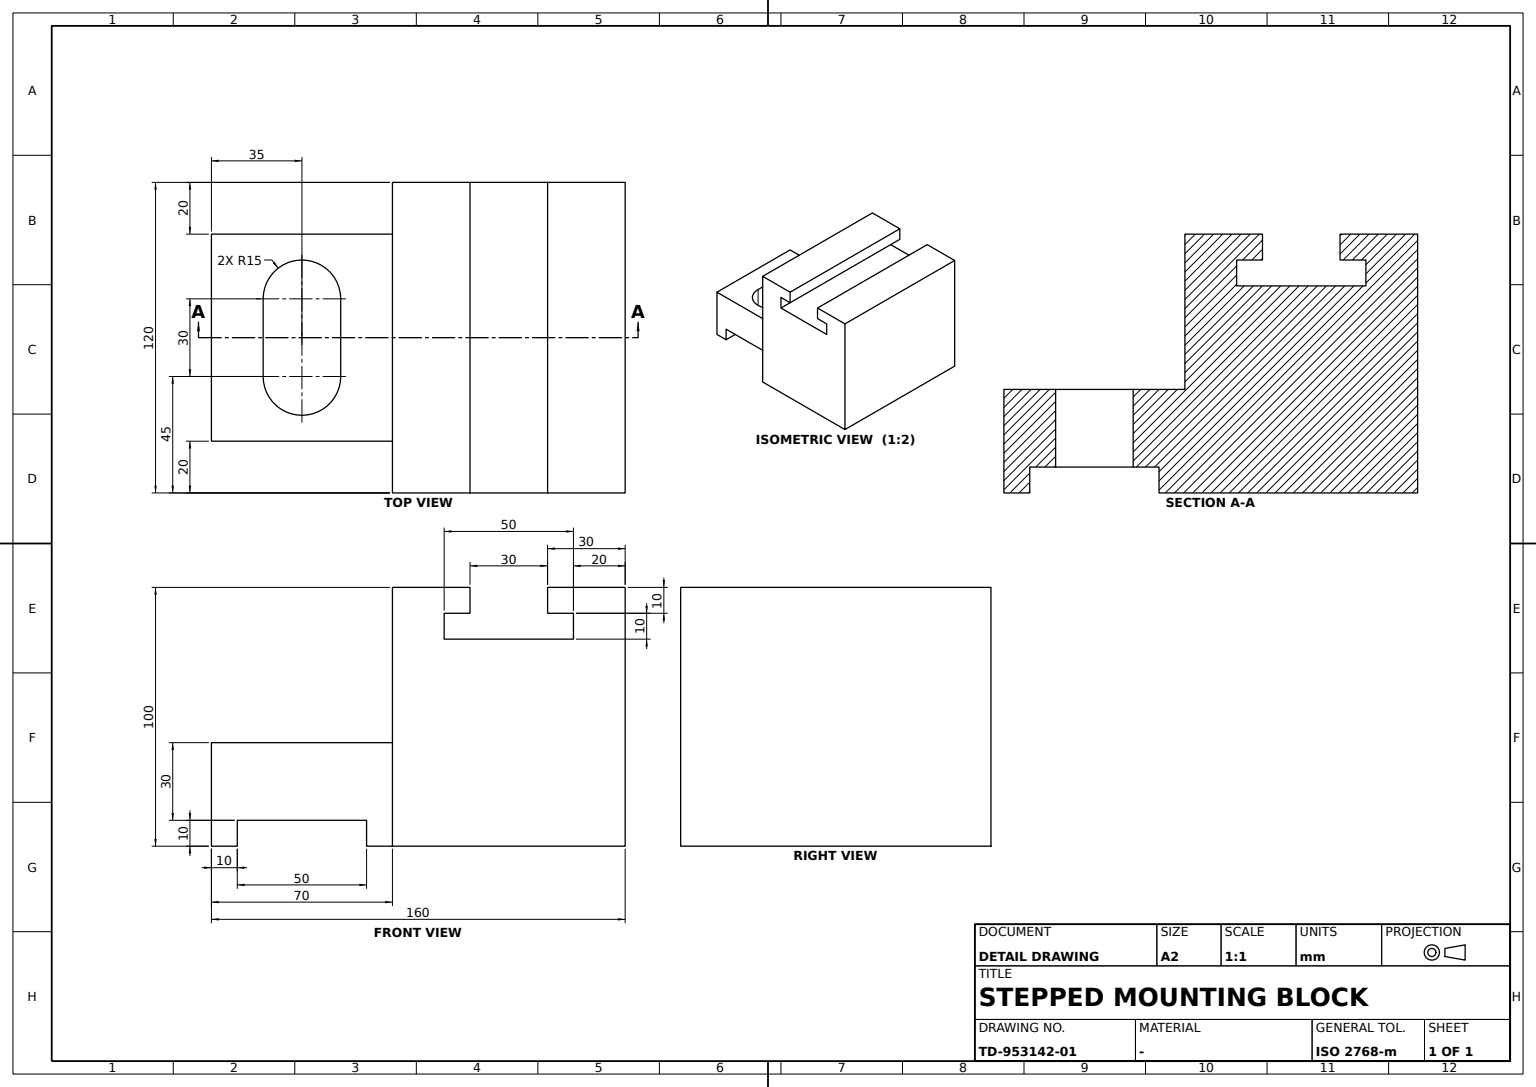
CATIA V5 part; units mm, degrees
sketch "Sketch1" plane through (0, 0, 0) normal (1, 0, 0) x (0, 1, 0)
  line L0 (0, 50) -> (0, -50)
  line L1 (0, 50) -> (90, 50)
  line L2 (90, 50) -> (90, -50)
  line L3 (90, -50) -> (0, -50)
  dimension "length L0" = 100
  dimension "length L1" = 90
  constraint midpoint L0 origin
  constraint vertical L0 y-axis
  constraint vertical L2 y-axis
  constraint horizontal L1 x-axis
  constraint horizontal L3 x-axis
extrude "Pad1" add sketch "Sketch1" along normal mid plane 120
sketch "Sketch2" plane through (0, 0, 0) normal (1, 0, 0) x (0, 1, 0)
  line L0 (0, 50) -> (0, -50) construction
  line L1 (0, -10) -> (0, -50)
  point P0 (0, -10)
  line L2 (0, -10) -> (-70, -10)
  line L3 (-70, -10) -> (-70, -50)
  point P1 (-70, -50)
  line L4 (0, -50) -> (-70, -50)
  point P2 (-70, -50)
  dimension "length L2" = 70
  dimension "length L3" = 40
  constraint coincidence P0 L0
  constraint coincidence P1 P2
  constraint vertical L3 y-axis
  constraint horizontal L2 x-axis
  constraint horizontal L4 x-axis
extrude "Pad2" add sketch "Sketch2" along normal blind 40 and the other way blind 40
sketch "Sketch3" plane through (60, 0, 0) normal (1, 0, 0) x (0, 1, 0)
  line L0 (30, 50) -> (60, 50)
  line L1 (90, 50) -> (0, 50) construction
  line L2 (30, 50) -> (30, 40)
  line L3 (30, 40) -> (20, 40)
  line L4 (20, 40) -> (20, 30)
  line L5 (20, 30) -> (70, 30)
  line L6 (70, 30) -> (70, 40)
  point P0 (70, 40)
  line L7 (70, 40) -> (60, 40)
  line L8 (60, 40) -> (60, 50)
  line L9 (90, -50) -> (90, 50) construction
  dimension "length L0" = 30
  dimension "length L2" = 10
  dimension "length L4" = 10
  dimension "length L5" = 50
  dimension "length L7" = 10
  dimension "distance L9 L6" = 20
  constraint horizontal L0 x-axis
  constraint horizontal L3 x-axis
  constraint horizontal L5 x-axis
  constraint horizontal L7 x-axis
  constraint coincidence L0 L1
  constraint coincidence P0 L3
  constraint vertical L2 y-axis
  constraint vertical L4 y-axis
  constraint vertical L6 y-axis
  constraint vertical L8 y-axis
extrude "Pocket1" cut sketch "Sketch3" against normal through all
sketch "Sketch4" plane through (40, 0, 0) normal (1, 0, 0) x (0, 1, 0)
  line L0 (-60, -40) -> (-10, -40)
  line L1 (-10, -40) -> (-10, -55.1789)
  line L2 (-10, -55.1789) -> (-60, -55.1789)
  line L3 (-60, -55.1789) -> (-60, -40)
  line L4 (0, 50) -> (0, -50) construction
  line L5 (0, -10) -> (-70, -10) construction
  dimension "length L2" = 50
  dimension "distance L4 L1" = 10
  dimension "distance L5 L0" = 30
  constraint horizontal L0 x-axis
  constraint horizontal L2 x-axis
  constraint vertical L1 y-axis
  constraint vertical L3 y-axis
extrude "Pocket2" cut sketch "Sketch4" against normal through all
sketch "Sketch5" plane through (0, 0, -10) normal (0, 0, 1) x (1, 0, 0)
  line L0 (-15, -35) -> (15, -35) construction
  point P0 (-15, -35)
  point P1 (15, -35)
  line L1 (-15, -20) -> (15, -20)
  line L2 (15, -50) -> (-15, -50)
  arc A0 (15, -20) -> (15, -50) centre (15, -35) cw
  arc A1 (-15, -50) -> (-15, -20) centre (-15, -35) cw
  line L3 (40, 0) -> (40, -70) construction
  dimension "distance L0 L1" = 15
  dimension "distance P0 P1" = 30
  dimension "distance origin L0" = 35
  dimension "distance P1 L3" = 25
  constraint horizontal L0 x-axis
  constraint tangency A0 L1
  constraint tangency A1 L1
  constraint tangency A0 L2
  constraint tangency A1 L2
extrude "Pocket3" cut sketch "Sketch5" against normal through all
sketch "Sketch6" plane through (0, 90, 0) normal (0, 1, 0) x (-1, 0, 0)
properties part number "Rectangular Mechanical Mounting Block with Slotted Hole and Stepped Profile"
